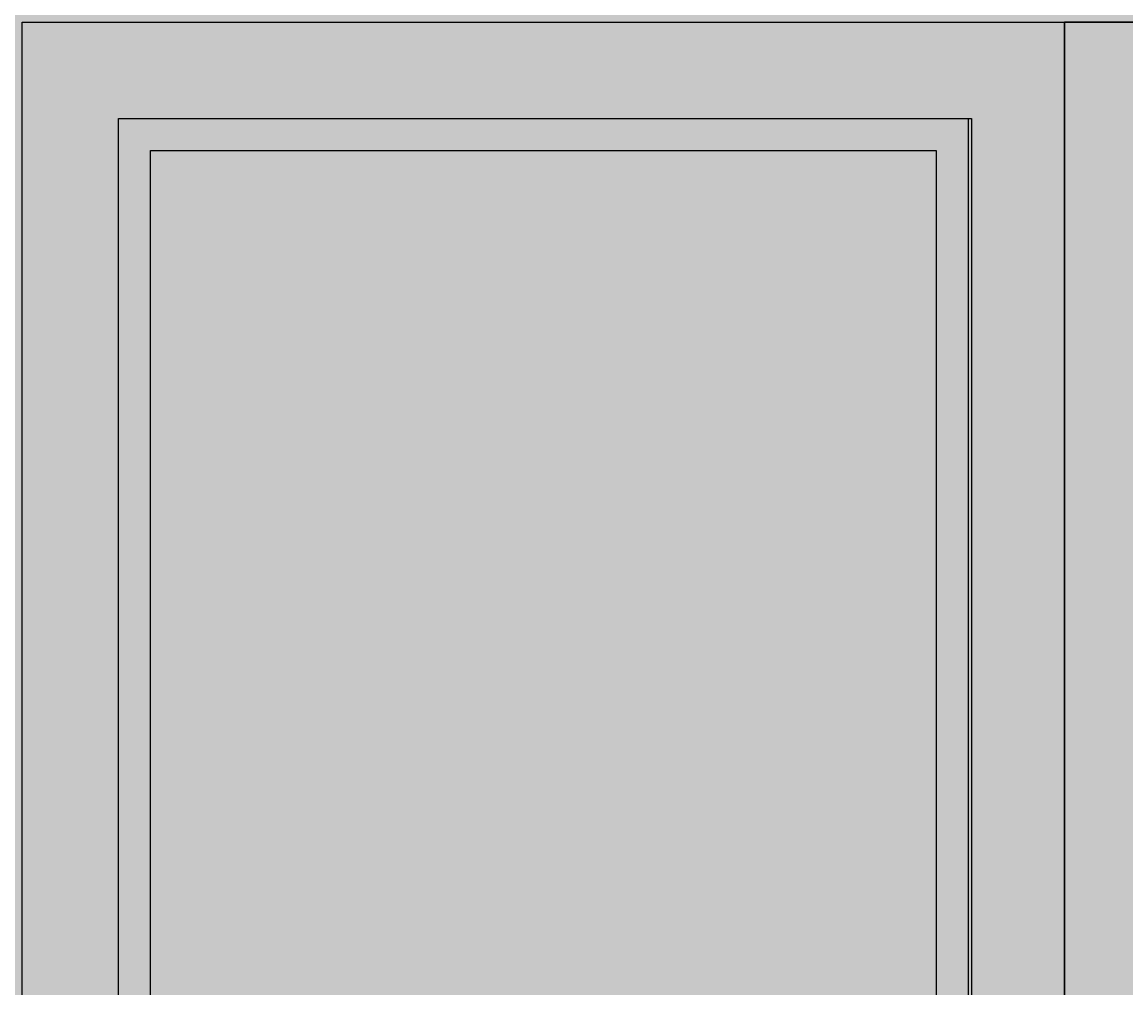
# Model space of a CAD drawing. Units: feet. Extents: x 2695 to 2912, y 795 to 1139.
# Tile 23 of 83: x 2774 to 2808, y 875 to 906. Entities that reach past the tile are written whole.
import ezdxf

# ---------------------------------------------------------------- set-up
doc = ezdxf.new("R2010")
doc.units = ezdxf.units.FT
for name, color, linetype, lineweight in [('A-ANNO-DIMS', 2, 'Continuous', 18), ('A-DOOR', 3, 'Continuous', 25), ('A-DOOR-PATT', 33, 'Continuous', 13), ('A-ELEV-PATT', 252, 'Continuous', 13)]:
    doc.layers.add(name, color=color, linetype=linetype, lineweight=lineweight)
doc.styles.get("Standard").update_dxf_attribs({"font": 'arial.ttf'})
doc.dimstyles.get("Standard").update_dxf_attribs({"dimtxt": 0.18, "dimasz": 0.18, "dimexe": 0.18, "dimexo": 0.0625, "dimgap": 0.09, "dimtad": 0, "dimtih": 1, "dimtoh": 1, "dimdec": 1, "dimzin": 0, "dimdsep": 46, "dimlunit": 3, "dimtxsty": 'Standard', "dimcen": 0.09, "dimadec": 0, "dimazin": 0, "dimtfac": 1, "dimtdec": 1, "dimtofl": 0, "dimtmove": 0, "dimatfit": 3, "dimfxl": 1, "dimtolj": 1, "dimtzin": 0, "dimarcsym": 0})

# ---------------------------------------------------------------- blocks, each defined once
blk = doc.blocks.new('*D14')
at = {"layer": 'A-ANNO-DIMS', "color": 0, "lineweight": -2, "transparency": 16777216}
for p, q in [((2838.439, 905.514), (2911.424, 905.514)), ((2911.244, 905.334), (2911.244, 890.368)), ((2911.244, 875.037), (2911.244, 890.004)), ((2758.214, 874.857), (2911.424, 874.857))]:
    blk.add_line(p, q, dxfattribs=at)
at = {"layer": 'A-ANNO-DIMS', "color": 0, "transparency": 16777216}
for points in [[(2911.214, 905.334), (2911.274, 905.334), (2911.244, 905.514)], [(2911.214, 875.037), (2911.274, 875.037), (2911.244, 874.857)]]:
    blk.add_solid(points, dxfattribs=at)
at = {"layer": 'Defpoints', "color": 0, "transparency": 16777216}
for p in [(2838.377, 905.514), (2911.244, 905.514), (2758.151, 874.857)]:
    blk.add_point(p, dxfattribs=at)
at = {"layer": 'A-ANNO-DIMS', "color": 0, "transparency": 16777216, "insert": (2911.244, 890.186), "char_height": 0.18, "attachment_point": 5}
blk.add_mtext('\\A1;30.66', dxfattribs=at)

msp = doc.modelspace()

# ---------------------------------------------------------------- hatches: boundary and pattern name
at = {"layer": 'A-DOOR-PATT'}
h = msp.add_hatch(color=256, dxfattribs=at)
h.set_gradient(color1=(211, 185, 150), color2=(211, 185, 150))
h.paths.add_polyline_path([(2805.9398, 905.5143), (2773.5029, 905.5143), (2773.5029, 810.9306), (2776.4999, 810.9306), (2776.4999, 902.5174), (2802.9429, 902.5174), (2802.9429, 810.9306), (2805.9398, 810.9306)])
h.paths.add_polyline_path([(2803.9681, 874.1057), (2805.0538, 874.1057), (2805.0538, 846.2857), (2803.9681, 846.2857)], flags=16)
h.paths.add_polyline_path([(2838.3767, 905.5143), (2805.9398, 905.5143), (2805.9398, 810.9306), (2808.9368, 810.9306), (2808.9368, 902.5174), (2835.3798, 902.5174), (2835.3798, 810.9306), (2838.3767, 810.9306)])
h = msp.add_hatch(color=256, dxfattribs=at)
h.set_gradient(color1=(211, 185, 150), color2=(211, 185, 150))
h.paths.add_polyline_path([(2777.5029, 901.5143), (2801.9398, 901.5143), (2801.9398, 810.9306), (2802.9429, 810.9306), (2802.9429, 902.5174), (2776.4999, 902.5174), (2776.4999, 810.9306), (2777.5029, 810.9306)])
h.paths.add_polyline_path([(2809.9398, 901.5143), (2834.3767, 901.5143), (2834.3767, 810.9306), (2835.3798, 810.9306), (2835.3798, 902.5174), (2808.9368, 902.5174), (2808.9368, 810.9306), (2809.9398, 810.9306)])
h = msp.add_hatch(color=256, dxfattribs=at)
h.set_gradient(color1=(173, 221, 247), color2=(173, 221, 247))
h.paths.add_polyline_path([(2801.9398, 901.5143), (2777.5029, 901.5143), (2777.5029, 810.9306), (2801.9398, 810.9306)])
h.paths.add_polyline_path([(2834.3767, 901.5143), (2809.9398, 901.5143), (2809.9398, 810.9306), (2834.3767, 810.9306)])
at = {"layer": 'A-ELEV-PATT'}
h = msp.add_hatch(color=256, dxfattribs=at)
h.set_gradient(color1=(147, 149, 152), color2=(147, 149, 152), tint=1)
h.paths.add_polyline_path([(2770.6361, 1118.4096), (2710.6361, 1118.4096), (2710.6361, 1062.9306), (2770.6361, 1062.9306)])
h.paths.add_polyline_path([(2890.6361, 1103.3378), (2770.6361, 1103.3378), (2770.6361, 1062.9306), (2890.6361, 1062.9306)])
h.paths.add_polyline_path([(2730.7081, 1048.1052), (2755.1125, 1048.1052), (2755.1125, 936.9306), (2770.6361, 936.9306), (2770.6361, 1050.3105), (2715.8852, 1050.3105), (2715.8852, 936.9306), (2730.7081, 936.9306)])
h.paths.add_polyline_path([(2890.6361, 1050.3105), (2770.6361, 1050.3105), (2770.6361, 971.9673), (2778.0341, 971.9673), (2778.0341, 1020.8235), (2843.575, 1020.8235), (2843.575, 971.9673), (2890.6361, 971.9673)])
h.paths.add_polyline_path([(2888.1882, 970.7156), (2843.575, 970.7156), (2843.575, 964.8267), (2888.1882, 964.8267)])
h.paths.add_polyline_path([(2888.1882, 964.1328), (2843.575, 964.1328), (2843.575, 956.614), (2888.1882, 956.614)])
h.paths.add_polyline_path([(2888.1882, 955.9202), (2843.575, 955.9202), (2843.575, 949.2892), (2888.1882, 949.2892)])
h.paths.add_polyline_path([(2888.1882, 948.5954), (2843.575, 948.5954), (2843.575, 941.3507), (2888.1882, 941.3507)])
h.paths.add_polyline_path([(2888.1882, 940.6569), (2843.575, 940.6569), (2843.575, 936.9306), (2888.1882, 936.9306)])
h.paths.add_polyline_path([(2890.6361, 970.7156), (2888.9368, 970.7156), (2888.9368, 964.8267), (2890.6361, 964.8267)])
h.paths.add_polyline_path([(2890.6361, 964.1328), (2888.9368, 964.1328), (2888.9368, 956.614), (2890.6361, 956.614)])
h.paths.add_polyline_path([(2890.6361, 955.9202), (2888.9368, 955.9202), (2888.9368, 949.2892), (2890.6361, 949.2892)])
h.paths.add_polyline_path([(2890.6361, 940.6569), (2888.9368, 940.6569), (2888.9368, 936.9306), (2890.6361, 936.9306)])
h.paths.add_polyline_path([(2890.6361, 948.5954), (2888.9368, 948.5954), (2888.9368, 941.3507), (2890.6361, 941.3507)])
h.paths.add_polyline_path([(2772.5216, 970.7156), (2770.6361, 970.7156), (2770.6361, 964.8267), (2772.5216, 964.8267)])
h.paths.add_polyline_path([(2772.5216, 964.1328), (2770.6361, 964.1328), (2770.6361, 956.614), (2772.5216, 956.614)])
h.paths.add_polyline_path([(2772.5216, 955.9202), (2770.6361, 955.9202), (2770.6361, 949.2892), (2772.5216, 949.2892)])
h.paths.add_polyline_path([(2772.5216, 948.5954), (2770.6361, 948.5954), (2770.6361, 941.3507), (2772.5216, 941.3507)])
h.paths.add_polyline_path([(2772.5216, 940.6569), (2770.6361, 940.6569), (2770.6361, 936.9306), (2772.5216, 936.9306)])
h.paths.add_polyline_path([(2778.0341, 940.6569), (2773.2702, 940.6569), (2773.2702, 936.9306), (2778.0341, 936.9306)])
h.paths.add_polyline_path([(2778.0341, 970.7156), (2773.2702, 970.7156), (2773.2702, 964.8267), (2778.0341, 964.8267)])
h.paths.add_polyline_path([(2778.0341, 964.1328), (2773.2702, 964.1328), (2773.2702, 956.614), (2778.0341, 956.614)])
h.paths.add_polyline_path([(2778.0341, 955.9202), (2773.2702, 955.9202), (2773.2702, 949.2892), (2778.0341, 949.2892)])
h.paths.add_polyline_path([(2778.0341, 948.5954), (2773.2702, 948.5954), (2773.2702, 941.3507), (2778.0341, 941.3507)])
h.paths.add_polyline_path([(2810.0407, 940.6569), (2780.0341, 940.6569), (2780.0341, 936.9306), (2810.0407, 936.9306)])
h.paths.add_polyline_path([(2890.6361, 924.3105), (2770.6361, 924.3105), (2770.6361, 810.9306), (2773.5029, 810.9306), (2773.5029, 905.5143), (2805.9398, 905.5143), (2838.3767, 905.5143), (2838.3767, 810.9306), (2890.6361, 810.9306)])

# ---------------------------------------------------------------- linework, layer by layer
at = {"layer": 'A-DOOR'}
for points in [[(2773.5029, 810.9306), (2773.5029, 905.5143), (2805.9398, 905.5143), (2805.9398, 810.9306)], [(2838.3767, 810.9306), (2838.3767, 905.5143), (2805.9398, 905.5143), (2805.9398, 810.9306)], [(2776.4999, 810.9306), (2776.4999, 902.5174), (2802.9429, 902.5174), (2802.9429, 810.9306)], [(2777.5029, 810.9306), (2777.5029, 901.5143), (2801.9398, 901.5143), (2801.9398, 810.9306)]]:
    msp.add_lwpolyline(points, dxfattribs=at)
for points in [[(2773.5029, 905.5143), (2838.3767, 905.5143), (2838.3767, 810.9306), (2773.5029, 810.9306)], [(2805.9398, 905.5143), (2805.9398, 905.5143), (2805.9398, 810.9306), (2805.9398, 810.9306)], [(2776.4999, 902.5174), (2803.0393, 902.5174), (2803.0393, 810.9306), (2776.4999, 810.9306)], [(2777.5029, 901.5143), (2801.9398, 901.5143), (2801.9398, 810.9306), (2777.5029, 810.9306)]]:
    msp.add_lwpolyline(points, close=True, dxfattribs=at)

# ---------------------------------------------------------------- dimensions: what is measured, and where the dimension line sits
at = {"layer": 'A-ANNO-DIMS'}
dim = msp.add_linear_dim(base=(2911.2444, 905.5143), p1=(2758.1515, 874.8571), p2=(2838.3767, 905.5143), angle=90, dimstyle='Standard', override={"dimdec": 2, "dimlfac": 1, "dimrnd": 0, "dimzin": 0, "dimdsep": 46, "dimlunit": 2}, dxfattribs=at)
dim.commit()
dim.dimension.update_dxf_attribs({"geometry": '*D14', "text_midpoint": (2911.2444, 890.1857)})

doc.saveas('drawing.dxf')
